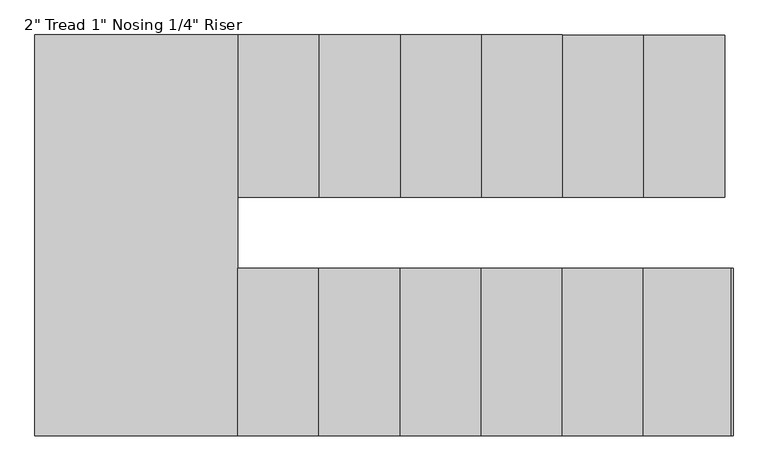
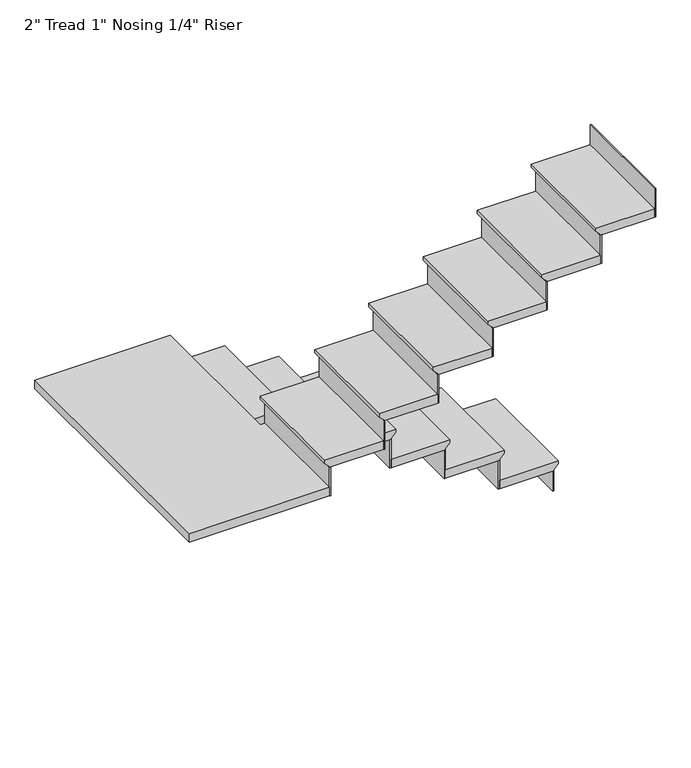
"""IFC4 building model written with IfcOpenShell, lengths in millimetres: stair flight geometry."""

from ifc_helpers import new_model, si_unit, origin, place, context, project, spatial, faceted_brep, source, transform, mapped, element, save


def stair_flight_79800fe3(model_context):
    return source(origin(), model_context, "Body", "Brep", [
        faceted_brep([(-2968.8120155, -2170.0065691, 150.2833333), (-2968.8120155, -2170.0065691, 169.3333333), (-2968.8120155, -2779.6065691, 169.3333333), (-2968.8120155, -2779.6065691, 150.2833333), (-2994.2120155, -2170.0065691, 124.8833333), (-2994.2120155, -2779.6065691, 124.8833333), (-3299.0120155, -2170.0065691, 169.3333333), (-3299.0120155, -2779.6065691, 169.3333333), (-2994.2120155, -2779.6065691, 118.5333333), (-3299.0120155, -2779.6065691, 118.5333333), (-3299.0120155, -2170.0065691, 118.5333333), (-2994.2120155, -2170.0065691, 118.5333333)], [[[0, 1, 2, 3]], [[4, 0, 3, 5]], [[2, 1, 6, 7]], [[8, 9, 10, 11]], [[2, 7, 9, 8, 5, 3]], [[8, 11, 4, 5]], [[6, 1, 0, 4, 11, 10]], [[7, 6, 10, 9]]]),
        faceted_brep([(-2994.2120155, -2170.0065691, 118.5333333), (-2994.2120155, -2170.0065691, 0.0), (-3000.5620155, -2170.0065691, 0.0), (-3000.5620155, -2170.0065691, 118.5333333), (-2994.2120155, -2779.6065691, 118.5333333), (-3000.5620155, -2779.6065691, 118.5333333), (-3000.5620155, -2779.6065691, 0.0), (-2994.2120155, -2779.6065691, 0.0)], [[[0, 1, 2, 3]], [[4, 5, 6, 7]], [[1, 0, 4, 7]], [[2, 1, 7, 6]], [[3, 2, 6, 5]], [[0, 3, 5, 4]]]),
        faceted_brep([(-3299.0120155, -2170.0065691, 287.8666667), (-3299.0120155, -2170.0065691, 118.5333333), (-3305.3620155, -2170.0065691, 118.5333333), (-3305.3620155, -2170.0065691, 287.8666667), (-3299.0120155, -2779.6065691, 287.8666667), (-3305.3620155, -2779.6065691, 287.8666667), (-3305.3620155, -2779.6065691, 118.5333333), (-3299.0120155, -2779.6065691, 118.5333333)], [[[0, 1, 2, 3]], [[4, 5, 6, 7]], [[1, 0, 4, 7]], [[2, 1, 7, 6]], [[3, 2, 6, 5]], [[0, 3, 5, 4]]]),
        faceted_brep([(-3273.6120155, -2779.6065691, 338.6666667), (-3273.6120155, -2170.0065691, 338.6666667), (-3603.8120155, -2170.0065691, 338.6666667), (-3603.8120155, -2779.6065691, 338.6666667), (-3299.0120155, -2779.6065691, 287.8666667), (-3603.8120155, -2779.6065691, 287.8666667), (-3603.8120155, -2170.0065691, 287.8666667), (-3299.0120155, -2170.0065691, 287.8666667), (-3299.0120155, -2779.6065691, 294.2166667), (-3273.6120155, -2779.6065691, 319.6166667), (-3299.0120155, -2170.0065691, 294.2166667), (-3273.6120155, -2170.0065691, 319.6166667)], [[[0, 1, 2, 3]], [[4, 5, 6, 7]], [[0, 3, 5, 4, 8, 9]], [[4, 7, 10, 8]], [[2, 1, 11, 10, 7, 6]], [[3, 2, 6, 5]], [[11, 1, 0, 9]], [[10, 11, 9, 8]]]),
        faceted_brep([(-3603.8120155, -2170.0065691, 457.2), (-3603.8120155, -2170.0065691, 287.8666667), (-3610.1620155, -2170.0065691, 287.8666667), (-3610.1620155, -2170.0065691, 457.2), (-3603.8120155, -2779.6065691, 457.2), (-3610.1620155, -2779.6065691, 457.2), (-3610.1620155, -2779.6065691, 287.8666667), (-3603.8120155, -2779.6065691, 287.8666667)], [[[0, 1, 2, 3]], [[4, 5, 6, 7]], [[1, 0, 4, 7]], [[2, 1, 7, 6]], [[3, 2, 6, 5]], [[0, 3, 5, 4]]]),
        faceted_brep([(-3578.4120155, -2779.6065691, 508.0), (-3578.4120155, -2170.0065691, 508.0), (-3908.6120155, -2170.0065691, 508.0), (-3908.6120155, -2779.6065691, 508.0), (-3603.8120155, -2779.6065691, 457.2), (-3908.6120155, -2779.6065691, 457.2), (-3908.6120155, -2170.0065691, 457.2), (-3603.8120155, -2170.0065691, 457.2), (-3603.8120155, -2779.6065691, 463.55), (-3578.4120155, -2779.6065691, 488.95), (-3603.8120155, -2170.0065691, 463.55), (-3578.4120155, -2170.0065691, 488.95)], [[[0, 1, 2, 3]], [[4, 5, 6, 7]], [[0, 3, 5, 4, 8, 9]], [[4, 7, 10, 8]], [[2, 1, 11, 10, 7, 6]], [[3, 2, 6, 5]], [[11, 1, 0, 9]], [[10, 11, 9, 8]]]),
        faceted_brep([(-3908.6120155, -2170.0065691, 626.5333333), (-3908.6120155, -2170.0065691, 457.2), (-3914.9620155, -2170.0065691, 457.2), (-3914.9620155, -2170.0065691, 626.5333333), (-3908.6120155, -2779.6065691, 626.5333333), (-3914.9620155, -2779.6065691, 626.5333333), (-3914.9620155, -2779.6065691, 457.2), (-3908.6120155, -2779.6065691, 457.2)], [[[0, 1, 2, 3]], [[4, 5, 6, 7]], [[1, 0, 4, 7]], [[2, 1, 7, 6]], [[3, 2, 6, 5]], [[0, 3, 5, 4]]]),
        faceted_brep([(-3883.2120155, -2779.6065691, 677.3333333), (-3883.2120155, -2170.0065691, 677.3333333), (-4213.4120155, -2170.0065691, 677.3333333), (-4213.4120155, -2779.6065691, 677.3333333), (-3908.6120155, -2779.6065691, 626.5333333), (-4213.4120155, -2779.6065691, 626.5333333), (-4213.4120155, -2170.0065691, 626.5333333), (-3908.6120155, -2170.0065691, 626.5333333), (-3908.6120155, -2779.6065691, 632.8833333), (-3883.2120155, -2779.6065691, 658.2833333), (-3908.6120155, -2170.0065691, 632.8833333), (-3883.2120155, -2170.0065691, 658.2833333)], [[[0, 1, 2, 3]], [[4, 5, 6, 7]], [[0, 3, 5, 4, 8, 9]], [[4, 7, 10, 8]], [[2, 1, 11, 10, 7, 6]], [[3, 2, 6, 5]], [[11, 1, 0, 9]], [[10, 11, 9, 8]]]),
        faceted_brep([(-4213.4120155, -2170.0065691, 795.8666667), (-4213.4120155, -2170.0065691, 626.5333333), (-4219.7620155, -2170.0065691, 626.5333333), (-4219.7620155, -2170.0065691, 795.8666667), (-4213.4120155, -2779.6065691, 795.8666667), (-4219.7620155, -2779.6065691, 795.8666667), (-4219.7620155, -2779.6065691, 626.5333333), (-4213.4120155, -2779.6065691, 626.5333333)], [[[0, 1, 2, 3]], [[4, 5, 6, 7]], [[1, 0, 4, 7]], [[2, 1, 7, 6]], [[3, 2, 6, 5]], [[0, 3, 5, 4]]]),
        faceted_brep([(-4188.0120155, -2779.6065691, 846.6666667), (-4188.0120155, -2170.0065691, 846.6666667), (-4518.2120155, -2170.0065691, 846.6666667), (-4518.2120155, -2779.6065691, 846.6666667), (-4213.4120155, -2779.6065691, 795.8666667), (-4518.2120155, -2779.6065691, 795.8666667), (-4518.2120155, -2170.0065691, 795.8666667), (-4213.4120155, -2170.0065691, 795.8666667), (-4213.4120155, -2779.6065691, 802.2166667), (-4188.0120155, -2779.6065691, 827.6166667), (-4213.4120155, -2170.0065691, 802.2166667), (-4188.0120155, -2170.0065691, 827.6166667)], [[[0, 1, 2, 3]], [[4, 5, 6, 7]], [[0, 3, 5, 4, 8, 9]], [[4, 7, 10, 8]], [[2, 1, 11, 10, 7, 6]], [[3, 2, 6, 5]], [[11, 1, 0, 9]], [[10, 11, 9, 8]]]),
        faceted_brep([(-4518.2120155, -2170.0065691, 965.2), (-4518.2120155, -2170.0065691, 795.8666667), (-4524.5620155, -2170.0065691, 795.8666667), (-4524.5620155, -2170.0065691, 965.2), (-4518.2120155, -2779.6065691, 965.2), (-4524.5620155, -2779.6065691, 965.2), (-4524.5620155, -2779.6065691, 795.8666667), (-4518.2120155, -2779.6065691, 795.8666667)], [[[0, 1, 2, 3]], [[4, 5, 6, 7]], [[1, 0, 4, 7]], [[2, 1, 7, 6]], [[3, 2, 6, 5]], [[0, 3, 5, 4]]]),
        faceted_brep([(-4492.8120155, -2779.6065691, 1016.0), (-4492.8120155, -2170.0065691, 1016.0), (-4823.0120155, -2170.0065691, 1016.0), (-4823.0120155, -2779.6065691, 1016.0), (-4518.2120155, -2779.6065691, 965.2), (-4823.0120155, -2779.6065691, 965.2), (-4823.0120155, -2170.0065691, 965.2), (-4518.2120155, -2170.0065691, 965.2), (-4518.2120155, -2779.6065691, 971.55), (-4492.8120155, -2779.6065691, 996.95), (-4518.2120155, -2170.0065691, 971.55), (-4492.8120155, -2170.0065691, 996.95)], [[[0, 1, 2, 3]], [[4, 5, 6, 7]], [[0, 3, 5, 4, 8, 9]], [[4, 7, 10, 8]], [[2, 1, 11, 10, 7, 6]], [[3, 2, 6, 5]], [[11, 1, 0, 9]], [[10, 11, 9, 8]]]),
        faceted_brep([(-4823.0120155, -2170.0065691, 1134.5333333), (-4823.0120155, -2170.0065691, 965.2), (-4829.3620155, -2170.0065691, 965.2), (-4829.3620155, -2170.0065691, 1134.5333333), (-4823.0120155, -2779.6065691, 1134.5333333), (-4829.3620155, -2779.6065691, 1134.5333333), (-4829.3620155, -2779.6065691, 965.2), (-4823.0120155, -2779.6065691, 965.2)], [[[0, 1, 2, 3]], [[4, 5, 6, 7]], [[1, 0, 4, 7]], [[2, 1, 7, 6]], [[3, 2, 6, 5]], [[0, 3, 5, 4]]]),
        faceted_brep([(-4772.2120155, -3046.3065691, 1185.3333333), (-4797.6120155, -3046.3065691, 1185.3333333), (-4797.6120155, -2170.0065691, 1185.3333333), (-5559.6120155, -2170.0065691, 1185.3333333), (-5559.6120155, -3674.9565691, 1185.3333333), (-4772.2120155, -3674.9565691, 1185.3333333), (-4797.6120155, -3046.3065691, 1134.5333333), (-4772.2120155, -3046.3065691, 1134.5333333), (-4772.2120155, -3674.9565691, 1134.5333333), (-5559.6120155, -3674.9565691, 1134.5333333), (-5559.6120155, -2170.0065691, 1134.5333333), (-4823.0120155, -2170.0065691, 1134.5333333), (-4823.0120155, -2779.6065691, 1134.5333333), (-4797.6120155, -2779.6065691, 1134.5333333), (-4797.6120155, -2779.6065691, 1166.2833333), (-4797.6120155, -2170.0065691, 1166.2833333), (-4823.0120155, -2779.6065691, 1140.8833333), (-4823.0120155, -2170.0065691, 1140.8833333)], [[[0, 1, 2, 3, 4, 5]], [[6, 7, 8, 9, 10, 11, 12, 13]], [[1, 0, 7, 6]], [[2, 1, 6, 13, 14, 15]], [[13, 12, 16, 14]], [[12, 11, 17, 16]], [[3, 2, 15, 17, 11, 10]], [[4, 3, 10, 9]], [[5, 4, 9, 8]], [[0, 5, 8, 7]], [[17, 15, 14, 16]]]),
        faceted_brep([(-4772.2120155, -3674.9565691, 1303.8666667), (-4772.2120155, -3674.9565691, 1134.5333333), (-4765.8620155, -3674.9565691, 1134.5333333), (-4765.8620155, -3674.9565691, 1303.8666667), (-4772.2120155, -3046.3065691, 1303.8666667), (-4765.8620155, -3046.3065691, 1303.8666667), (-4765.8620155, -3046.3065691, 1134.5333333), (-4772.2120155, -3046.3065691, 1134.5333333)], [[[0, 1, 2, 3]], [[4, 5, 6, 7]], [[1, 0, 4, 7]], [[2, 1, 7, 6]], [[3, 2, 6, 5]], [[0, 3, 5, 4]]]),
        faceted_brep([(-4797.6120155, -3046.3065691, 1354.6666667), (-4797.6120155, -3674.9565691, 1354.6666667), (-4467.4120155, -3674.9565691, 1354.6666667), (-4467.4120155, -3046.3065691, 1354.6666667), (-4772.2120155, -3046.3065691, 1303.8666667), (-4467.4120155, -3046.3065691, 1303.8666667), (-4467.4120155, -3674.9565691, 1303.8666667), (-4772.2120155, -3674.9565691, 1303.8666667), (-4772.2120155, -3046.3065691, 1310.2166667), (-4797.6120155, -3046.3065691, 1335.6166667), (-4772.2120155, -3674.9565691, 1310.2166667), (-4797.6120155, -3674.9565691, 1335.6166667)], [[[0, 1, 2, 3]], [[4, 5, 6, 7]], [[0, 3, 5, 4, 8, 9]], [[4, 7, 10, 8]], [[2, 1, 11, 10, 7, 6]], [[3, 2, 6, 5]], [[11, 1, 0, 9]], [[10, 11, 9, 8]]]),
        faceted_brep([(-4467.4120155, -3674.9565691, 1473.2), (-4467.4120155, -3674.9565691, 1303.8666667), (-4461.0620155, -3674.9565691, 1303.8666667), (-4461.0620155, -3674.9565691, 1473.2), (-4467.4120155, -3046.3065691, 1473.2), (-4461.0620155, -3046.3065691, 1473.2), (-4461.0620155, -3046.3065691, 1303.8666667), (-4467.4120155, -3046.3065691, 1303.8666667)], [[[0, 1, 2, 3]], [[4, 5, 6, 7]], [[1, 0, 4, 7]], [[2, 1, 7, 6]], [[3, 2, 6, 5]], [[0, 3, 5, 4]]]),
        faceted_brep([(-4492.8120155, -3046.3065691, 1524.0), (-4492.8120155, -3674.9565691, 1524.0), (-4162.6120155, -3674.9565691, 1524.0), (-4162.6120155, -3046.3065691, 1524.0), (-4467.4120155, -3046.3065691, 1473.2), (-4162.6120155, -3046.3065691, 1473.2), (-4162.6120155, -3674.9565691, 1473.2), (-4467.4120155, -3674.9565691, 1473.2), (-4467.4120155, -3046.3065691, 1479.55), (-4492.8120155, -3046.3065691, 1504.95), (-4467.4120155, -3674.9565691, 1479.55), (-4492.8120155, -3674.9565691, 1504.95)], [[[0, 1, 2, 3]], [[4, 5, 6, 7]], [[0, 3, 5, 4, 8, 9]], [[4, 7, 10, 8]], [[2, 1, 11, 10, 7, 6]], [[3, 2, 6, 5]], [[11, 1, 0, 9]], [[10, 11, 9, 8]]]),
        faceted_brep([(-4162.6120155, -3674.9565691, 1642.5333333), (-4162.6120155, -3674.9565691, 1473.2), (-4156.2620155, -3674.9565691, 1473.2), (-4156.2620155, -3674.9565691, 1642.5333333), (-4162.6120155, -3046.3065691, 1642.5333333), (-4156.2620155, -3046.3065691, 1642.5333333), (-4156.2620155, -3046.3065691, 1473.2), (-4162.6120155, -3046.3065691, 1473.2)], [[[0, 1, 2, 3]], [[4, 5, 6, 7]], [[1, 0, 4, 7]], [[2, 1, 7, 6]], [[3, 2, 6, 5]], [[0, 3, 5, 4]]]),
        faceted_brep([(-4188.0120155, -3046.3065691, 1693.3333333), (-4188.0120155, -3674.9565691, 1693.3333333), (-3857.8120155, -3674.9565691, 1693.3333333), (-3857.8120155, -3046.3065691, 1693.3333333), (-4162.6120155, -3046.3065691, 1642.5333333), (-3857.8120155, -3046.3065691, 1642.5333333), (-3857.8120155, -3674.9565691, 1642.5333333), (-4162.6120155, -3674.9565691, 1642.5333333), (-4162.6120155, -3046.3065691, 1648.8833333), (-4188.0120155, -3046.3065691, 1674.2833333), (-4162.6120155, -3674.9565691, 1648.8833333), (-4188.0120155, -3674.9565691, 1674.2833333)], [[[0, 1, 2, 3]], [[4, 5, 6, 7]], [[0, 3, 5, 4, 8, 9]], [[4, 7, 10, 8]], [[2, 1, 11, 10, 7, 6]], [[3, 2, 6, 5]], [[11, 1, 0, 9]], [[10, 11, 9, 8]]]),
        faceted_brep([(-3857.8120155, -3674.9565691, 1811.8666667), (-3857.8120155, -3674.9565691, 1642.5333333), (-3851.4620155, -3674.9565691, 1642.5333333), (-3851.4620155, -3674.9565691, 1811.8666667), (-3857.8120155, -3046.3065691, 1811.8666667), (-3851.4620155, -3046.3065691, 1811.8666667), (-3851.4620155, -3046.3065691, 1642.5333333), (-3857.8120155, -3046.3065691, 1642.5333333)], [[[0, 1, 2, 3]], [[4, 5, 6, 7]], [[1, 0, 4, 7]], [[2, 1, 7, 6]], [[3, 2, 6, 5]], [[0, 3, 5, 4]]]),
        faceted_brep([(-3883.2120155, -3046.3065691, 1862.6666667), (-3883.2120155, -3674.9565691, 1862.6666667), (-3553.0120155, -3674.9565691, 1862.6666667), (-3553.0120155, -3046.3065691, 1862.6666667), (-3857.8120155, -3046.3065691, 1811.8666667), (-3553.0120155, -3046.3065691, 1811.8666667), (-3553.0120155, -3674.9565691, 1811.8666667), (-3857.8120155, -3674.9565691, 1811.8666667), (-3857.8120155, -3046.3065691, 1818.2166667), (-3883.2120155, -3046.3065691, 1843.6166667), (-3857.8120155, -3674.9565691, 1818.2166667), (-3883.2120155, -3674.9565691, 1843.6166667)], [[[0, 1, 2, 3]], [[4, 5, 6, 7]], [[0, 3, 5, 4, 8, 9]], [[4, 7, 10, 8]], [[2, 1, 11, 10, 7, 6]], [[3, 2, 6, 5]], [[11, 1, 0, 9]], [[10, 11, 9, 8]]]),
        faceted_brep([(-3553.0120155, -3674.9565691, 1981.2), (-3553.0120155, -3674.9565691, 1811.8666667), (-3546.6620155, -3674.9565691, 1811.8666667), (-3546.6620155, -3674.9565691, 1981.2), (-3553.0120155, -3046.3065691, 1981.2), (-3546.6620155, -3046.3065691, 1981.2), (-3546.6620155, -3046.3065691, 1811.8666667), (-3553.0120155, -3046.3065691, 1811.8666667)], [[[0, 1, 2, 3]], [[4, 5, 6, 7]], [[1, 0, 4, 7]], [[2, 1, 7, 6]], [[3, 2, 6, 5]], [[0, 3, 5, 4]]]),
        faceted_brep([(-3578.4120155, -3046.3065691, 2032.0), (-3578.4120155, -3674.9565691, 2032.0), (-3248.2120155, -3674.9565691, 2032.0), (-3248.2120155, -3046.3065691, 2032.0), (-3553.0120155, -3046.3065691, 1981.2), (-3248.2120155, -3046.3065691, 1981.2), (-3248.2120155, -3674.9565691, 1981.2), (-3553.0120155, -3674.9565691, 1981.2), (-3553.0120155, -3046.3065691, 1987.55), (-3578.4120155, -3046.3065691, 2012.95), (-3553.0120155, -3674.9565691, 1987.55), (-3578.4120155, -3674.9565691, 2012.95)], [[[0, 1, 2, 3]], [[4, 5, 6, 7]], [[0, 3, 5, 4, 8, 9]], [[4, 7, 10, 8]], [[2, 1, 11, 10, 7, 6]], [[3, 2, 6, 5]], [[11, 1, 0, 9]], [[10, 11, 9, 8]]]),
        faceted_brep([(-3248.2120155, -3674.9565691, 2150.5333333), (-3248.2120155, -3674.9565691, 1981.2), (-3241.8620155, -3674.9565691, 1981.2), (-3241.8620155, -3674.9565691, 2150.5333333), (-3248.2120155, -3046.3065691, 2150.5333333), (-3241.8620155, -3046.3065691, 2150.5333333), (-3241.8620155, -3046.3065691, 1981.2), (-3248.2120155, -3046.3065691, 1981.2)], [[[0, 1, 2, 3]], [[4, 5, 6, 7]], [[1, 0, 4, 7]], [[2, 1, 7, 6]], [[3, 2, 6, 5]], [[0, 3, 5, 4]]]),
        faceted_brep([(-2943.4120155, -3674.9565691, 2319.8666667), (-2943.4120155, -3674.9565691, 2150.5333333), (-2937.0620155, -3674.9565691, 2150.5333333), (-2937.0620155, -3674.9565691, 2319.8666667), (-2943.4120155, -3046.3065691, 2319.8666667), (-2937.0620155, -3046.3065691, 2319.8666667), (-2937.0620155, -3046.3065691, 2150.5333333), (-2943.4120155, -3046.3065691, 2150.5333333)], [[[0, 1, 2, 3]], [[4, 5, 6, 7]], [[1, 0, 4, 7]], [[2, 1, 7, 6]], [[3, 2, 6, 5]], [[0, 3, 5, 4]]]),
        faceted_brep([(-3273.6120155, -3046.3065691, 2201.3333333), (-3273.6120155, -3674.9565691, 2201.3333333), (-2943.4120155, -3674.9565691, 2201.3333333), (-2943.4120155, -3046.3065691, 2201.3333333), (-3248.2120155, -3046.3065691, 2150.5333333), (-2943.4120155, -3046.3065691, 2150.5333333), (-2943.4120155, -3674.9565691, 2150.5333333), (-3248.2120155, -3674.9565691, 2150.5333333), (-3248.2120155, -3046.3065691, 2156.8833333), (-3273.6120155, -3046.3065691, 2182.2833333), (-3248.2120155, -3674.9565691, 2156.8833333), (-3273.6120155, -3674.9565691, 2182.2833333)], [[[0, 1, 2, 3]], [[4, 5, 6, 7]], [[0, 3, 5, 4, 8, 9]], [[4, 7, 10, 8]], [[2, 1, 11, 10, 7, 6]], [[3, 2, 6, 5]], [[11, 1, 0, 9]], [[10, 11, 9, 8]]]),
    ])


if __name__ == "__main__":
    model = new_model("IFC4")
    model_context = context("Model", 3, world=origin())
    ifc_project = project(units=[si_unit("LENGTHUNIT", "METRE", prefix="MILLI")], contexts=[model_context])
    site = spatial("IfcSite", under=ifc_project)
    building = spatial("IfcBuilding", under=site)
    placement = place(None, origin())
    stair_flight_shape = stair_flight_79800fe3(model_context)
    element("IfcStairFlight", 1, ObjectType="2\" Tread 1\" Nosing 1/4\" Riser", at=placement, inside=building, context=model_context, shape_type="MappedRepresentation", body=[
        mapped(stair_flight_shape, transform((0.0, 0.0, 0.0), x_axis=(1.0, 0.0, 0.0), y_axis=(0.0, 1.0, 0.0), z_axis=(0.0, 0.0, 1.0))),
    ])
    save(model, "model.ifc")
